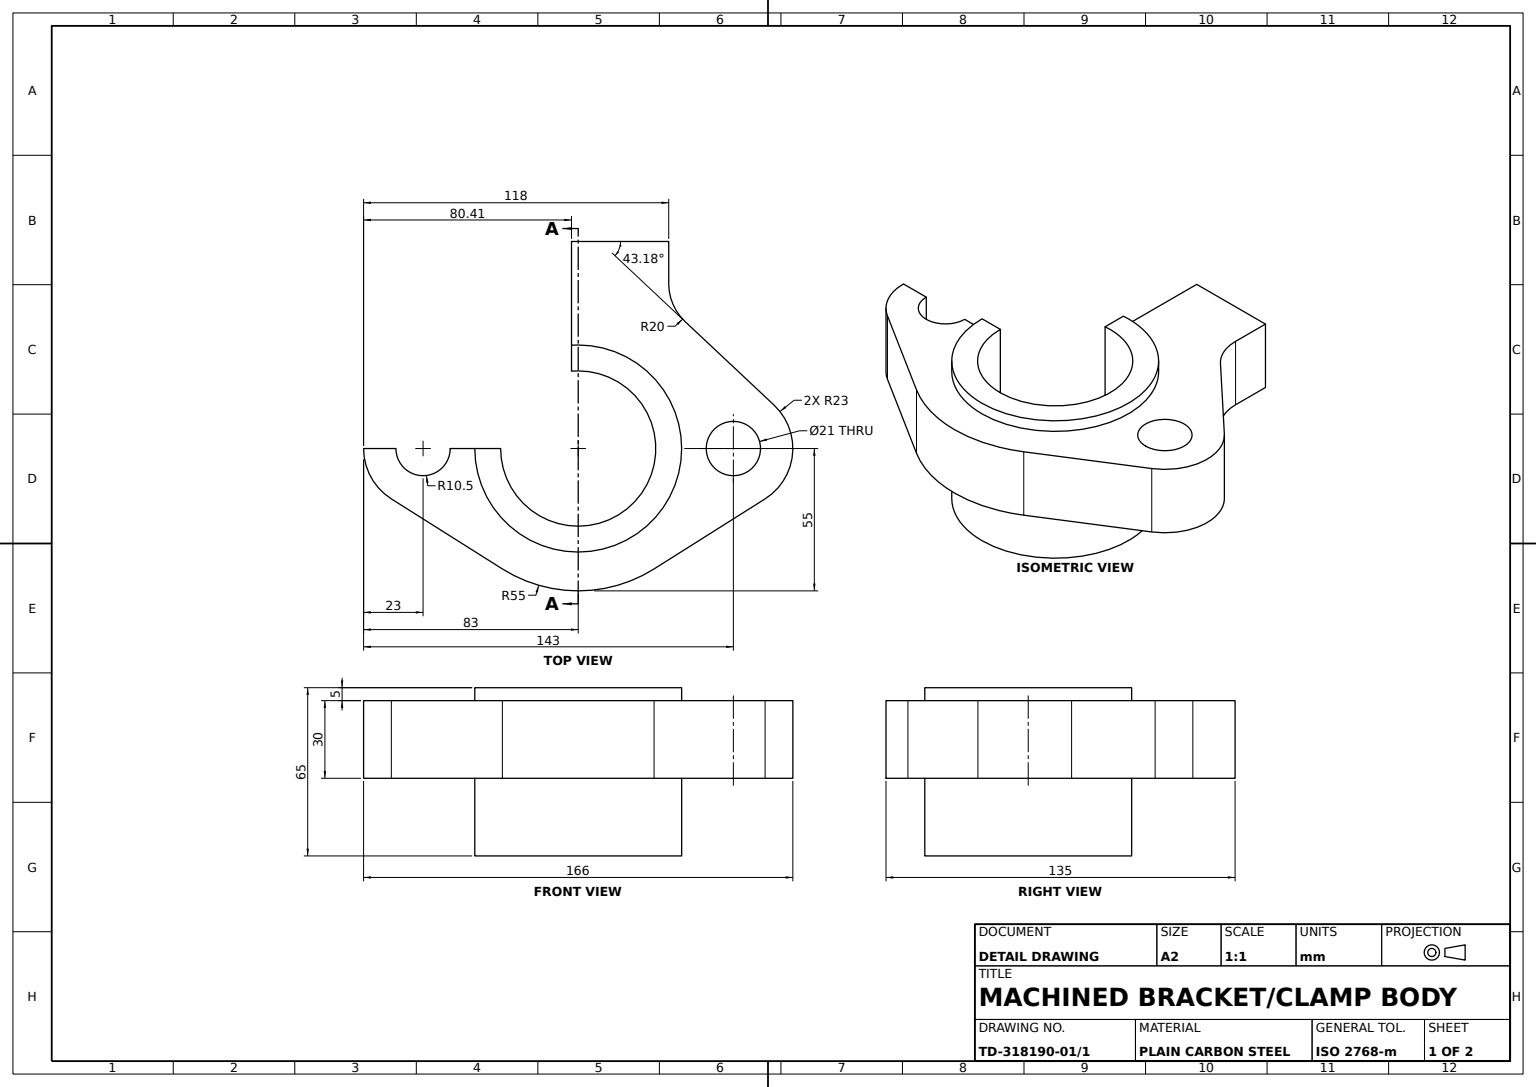
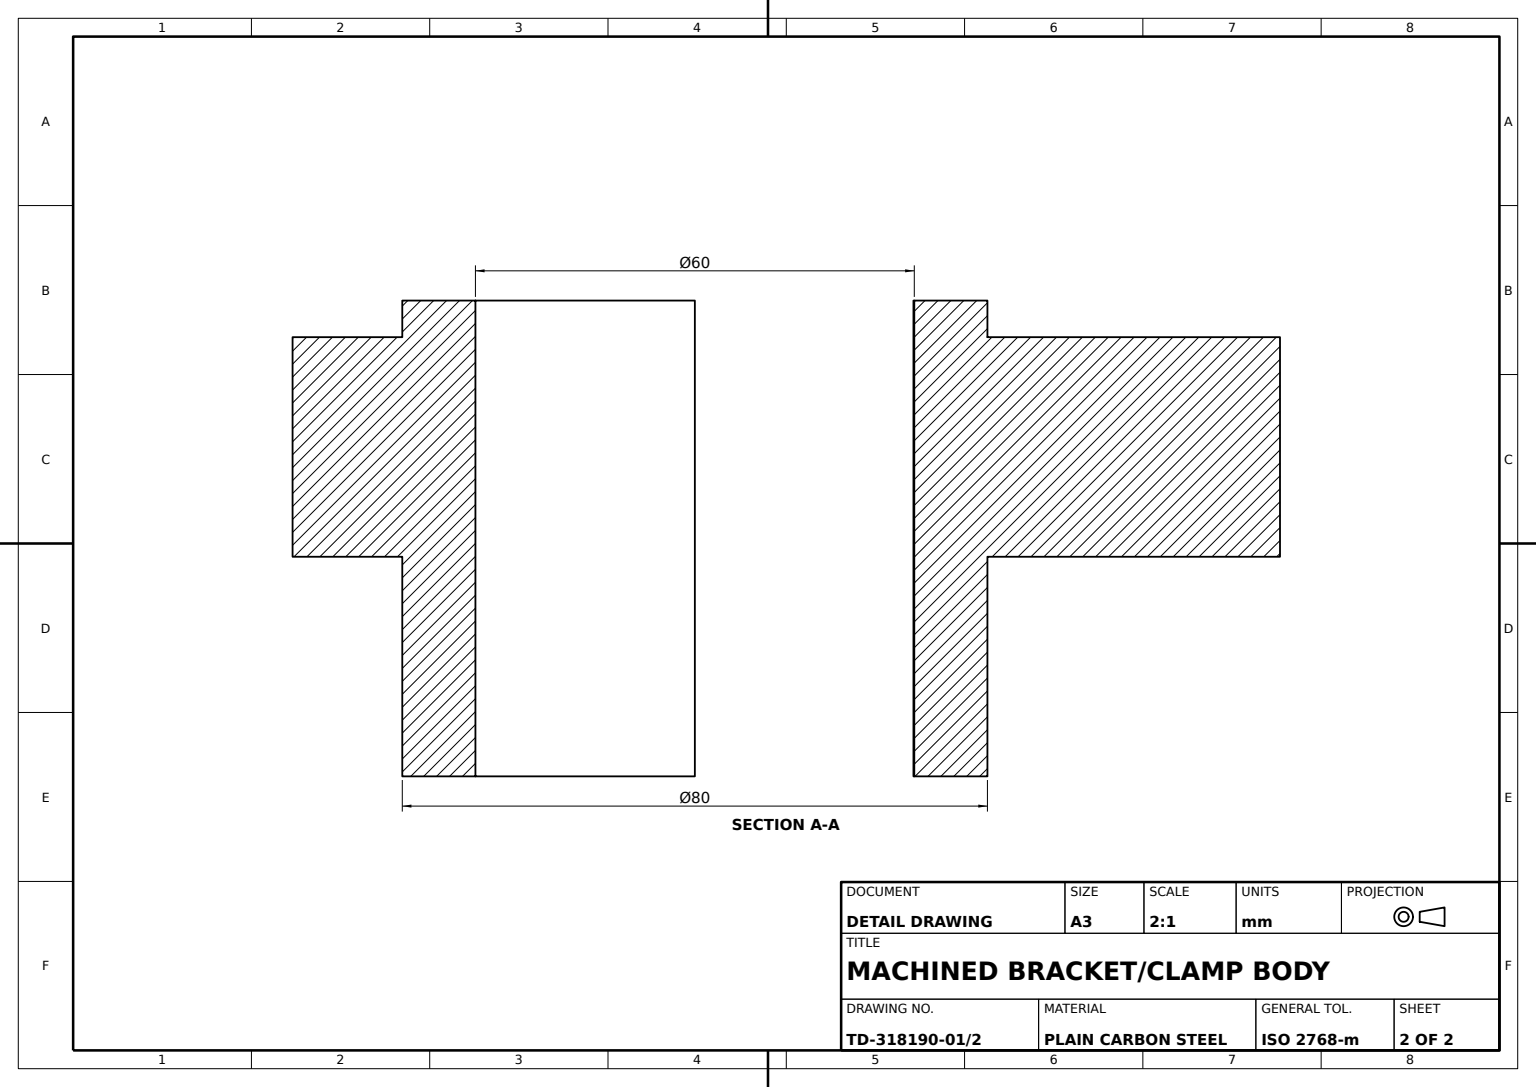
SolidWorks part; units mm, degrees
material "Plain Carbon Steel"
ref_plane "Front Plane" through (0, 0, 0) normal (0, 0, 1) x (1, 0, 0)
ref_plane "Top Plane" through (0, 0, 0) normal (0, 1, 0) x (1, 0, 0)
ref_plane "Right Plane" through (0, 0, 0) normal (1, 0, 0) x (0, 0, -1)
sketch "Hub Tube Sketch" plane through (0, 0, 0) normal (0, 1, 0) x (1, 0, 0)
  circle A0 centre (0, 0) radius 30
  circle A1 centre (0, 0) radius 40
  dimension "D1" = 60
  dimension "D2" = 80
extrude "Hub Tube Ø80" add sketch "Hub Tube Sketch" along normal mid plane 60
sketch "Flange Profile Sketch" plane through (0, 30, 0) normal (0, 1, 0) x (1, 0, 0)
  line L0 (-72.2667, -19.4558) -> (-29.3333, -46.5248)
  line L1 (29.3333, -46.5248) -> (72.2667, -19.4558)
  line L2 (0, 0) -> (0, 73.8367)
  line L5 (-35, 63.6591) -> (-35, 80)
  line L6 (-35, 80) -> (35, 80)
  line L7 (35, 80) -> (35, 63.6591)
  line L8 (-41.3144, 49.0747) -> (-75.7385, 16.772)
  line L9 (41.3144, 49.0747) -> (75.7385, 16.772)
  arc A1 (72.2667, -19.4558) -> (75.7385, 16.772) centre (60, 0) ccw
  arc A2 (-75.7385, 16.772) -> (-72.2667, -19.4558) centre (-60, 0) ccw
  arc A7 (-41.3144, 49.0747) -> (-35, 63.6591) centre (-55, 63.6591) ccw
  arc A8 (-29.3333, -46.5248) -> (29.3333, -46.5248) centre (0, 0) ccw
  arc A9 (35, 63.6591) -> (41.3144, 49.0747) centre (55, 63.6591) ccw
  point P4 (-35, 55)
  dimension "D1" = 46
  dimension "D2" = 20
  dimension "D3" = 46
  dimension "D4" = 20
  dimension "D5" = 35
  dimension "D11" = 55
  dimension "D6" = 60
  dimension "D7" = 60
  dimension "D8" = 70
  dimension "D9" = 80
  dimension "D10" = 25
  dimension "D12" = 73.8367
extrude "Flange 30mm" add sketch "Flange Profile Sketch" against normal blind 30
sketch "Collar Sketch" plane through (0, 30, 0) normal (0, 1, 0) x (1, 0, 0)
  circle A0 centre (0, 0) radius 40
  circle A1 centre (0, 0) radius 30
  dimension "D1" = 80
  dimension "D2" = 60
extrude "Collar Ø80 x5" add sketch "Collar Sketch" along normal blind 5
sketch "Side Slot Sketch" plane through (0, 0, 0) normal (0, -1, 0) x (1, 0, 0)
  line L0 (0, 0) -> (-5.1861, 0)
  line L1 (-109.1614, 0) -> (-2.5931, 0)
  line L2 (-2.5931, 0) -> (-2.5931, -87.1295)
  line L3 (-2.5931, -87.1295) -> (-109.1614, -88.9003)
  line L4 (-109.1614, -88.9003) -> (-109.1614, 0)
  arc M7 (-72.2667, 19.4558) -> (-75.7385, -16.772) centre (-60, 0) ccw
  line M8 (-75.7385, -16.772) -> (-41.3144, -49.0747)
  arc M9 (-41.3144, -49.0747) -> (-35, -63.6591) centre (-55, -63.6591) cw
  line M10 (-35, -63.6591) -> (-35, -80)
  line M11 (-35, -80) -> (35, -80)
  circle M13 centre (0, 0) radius 40
  dimension "D1" = 70.5523
  dimension "D2" = 33.423
  dimension "D3" = 38.0547
  dimension "D4" = 39.8256
extrude "Side Slot Cut" cut sketch "Side Slot Sketch" against normal blind 140 and the other way blind 135 contours L2 L1 M13 M7 M8 M9 M10 M11 | L2 L0 L1 M13 | L4 L3 L2 L1 M11 M10 M9 M8 M7
sketch "Cut Ø21 A Sketch" plane through (0, 0, 0) normal (0, -1, 0) x (1, 0, 0)
  circle A0 centre (60, 0) radius 10.5
  dimension "D1" = 21
extrude "Cut Ø21 A" cut sketch "Cut Ø21 A Sketch" against normal blind 159 and the other way blind 99
sketch "Cut Ø21 B Sketch" plane through (0, 0, 0) normal (0, -1, 0) x (1, 0, 0)
  circle A0 centre (-60, 0) radius 10.5
  dimension "D1" = 21
extrude "Cut Ø21 B" cut sketch "Cut Ø21 B Sketch" against normal blind 405 and the other way blind 507
